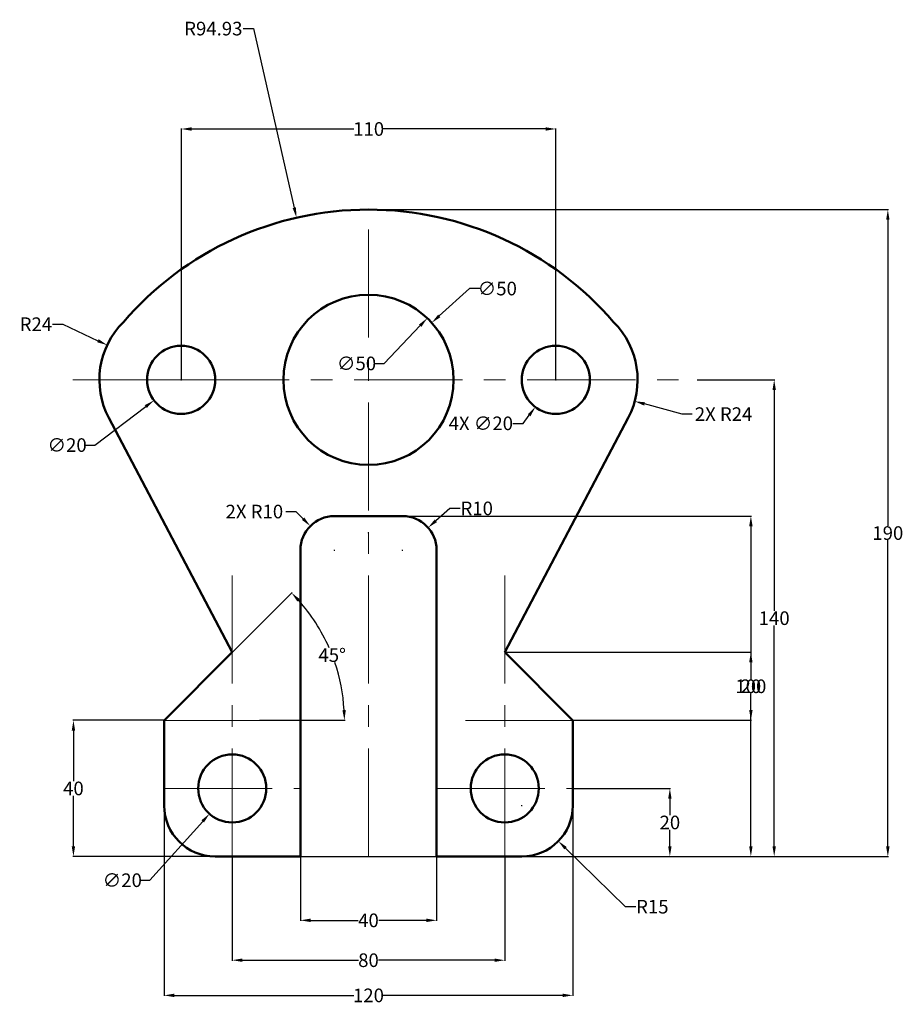
# Model space of a CAD drawing. Units: inches. Extents: x 304 to 564, y 197 to 487.
import ezdxf

# ---------------------------------------------------------------- set-up
doc = ezdxf.new("R2010")
doc.units = ezdxf.units.IN
doc.header["$MEASUREMENT"] = 0
doc.linetypes.add('CENTER', pattern=[50.8, 31.75, -6.35, 6.35, -6.35])
for name, color, linetype, lineweight in [('M-CNTR', 4, 'CENTER', 18), ('M-CONS', 8, 'Continuous', 13), ('M-DIMS', 2, 'Continuous', 25), ('M-OUTL', 7, 'Continuous', 50)]:
    doc.layers.add(name, color=color, linetype=linetype, lineweight=lineweight)
doc.styles.get("Standard").update_dxf_attribs({"font": 'arial.ttf'})
doc.dimstyles.get("Standard").update_dxf_attribs({"dimtxt": 4, "dimasz": 3, "dimexe": 0.18, "dimexo": 0.0625, "dimgap": 0.09, "dimtad": 0, "dimtih": 1, "dimtoh": 1, "dimdec": 0, "dimzin": 0, "dimdsep": 46, "dimtxsty": 'Standard', "dimcen": 0.09, "dimadec": 0, "dimazin": 0, "dimtfac": 1, "dimtdec": 0, "dimtofl": 0, "dimtmove": 0, "dimatfit": 3, "dimfxl": 1, "dimtolj": 1, "dimtzin": 0, "dimarcsym": 0})

# ---------------------------------------------------------------- blocks, each defined once
blk = doc.blocks.new('*D1')
at = {"layer": 'Defpoints', "color": 0, "transparency": 16777216}
for p in [(386.62, 240.9), (426.62, 240.9), (426.62, 222.16)]:
    blk.add_point(p, dxfattribs=at)
at = {"layer": 'M-DIMS', "color": 0, "lineweight": -2, "transparency": 16777216}
for p, q in [((386.62, 240.84), (386.62, 221.98)), ((426.62, 240.84), (426.62, 221.98)), ((389.62, 222.16), (403.6, 222.16)), ((423.62, 222.16), (409.65, 222.16))]:
    blk.add_line(p, q, dxfattribs=at)
at = {"layer": 'M-DIMS', "color": 0, "transparency": 16777216}
for points in [[(389.62, 222.66), (389.62, 221.66), (386.62, 222.16)], [(423.62, 222.66), (423.62, 221.66), (426.62, 222.16)]]:
    blk.add_solid(points, dxfattribs=at)
at = {"layer": 'M-DIMS', "color": 0, "transparency": 16777216, "insert": (406.62, 222.16), "char_height": 4, "attachment_point": 5}
blk.add_mtext('\\A1;40', dxfattribs=at)
blk = doc.blocks.new('*D2')
at = {"layer": 'Defpoints', "color": 0, "transparency": 16777216}
for p in [(392.46, 307.36), (366.62, 300.9), (346.62, 280.9), (346.62, 280.9), (374.57, 280.9)]:
    blk.add_point(p, dxfattribs=at)
at = {"layer": 'M-DIMS', "color": 0, "lineweight": -2, "transparency": 16777216}
for p, q in [((366.67, 300.94), (384.18, 318.45)), ((374.64, 280.9), (399.73, 280.9))]:
    blk.add_line(p, q, dxfattribs=at)
for start, end in [(23.6991, 41.7521), (3.2479, 18.764)]:
    blk.add_arc((346.62, 280.9), 52.93, start, end, dxfattribs=at)
at = {"layer": 'M-DIMS', "color": 0, "transparency": 16777216}
for points in [[(385.75, 315.8), (386.48, 316.49), (384.05, 318.33)], [(399.97, 283.91), (398.97, 283.88), (399.55, 280.9)]]:
    blk.add_solid(points, dxfattribs=at)
at = {"layer": 'M-DIMS', "color": 0, "transparency": 16777216, "insert": (395.97, 300.05), "char_height": 4, "attachment_point": 5}
blk.add_mtext('\\A1;45°', dxfattribs=at)
blk = doc.blocks.new('*D3')
at = {"layer": 'Defpoints', "color": 0, "transparency": 16777216}
for p in [(373.3, 268.34), (359.95, 253.45)]:
    blk.add_point(p, dxfattribs=at)
at = {"layer": 'M-DIMS', "color": 0, "lineweight": -2, "transparency": 16777216}
for p, q in [((366.53, 260.9), (366.71, 260.9)), ((366.62, 260.81), (366.62, 260.99)), ((342.47, 233.95), (357.95, 251.22)), ((339.47, 233.95), (342.47, 233.95))]:
    blk.add_line(p, q, dxfattribs=at)
at = {"layer": 'M-DIMS', "color": 0, "transparency": 16777216}
blk.add_solid([(357.57, 251.55), (358.32, 250.89), (359.95, 253.45)], dxfattribs=at)
at = {"layer": 'M-DIMS', "color": 0, "transparency": 16777216, "insert": (334.34, 233.95), "char_height": 4, "attachment_point": 5}
blk.add_mtext('\\A1;∅20', dxfattribs=at)
blk = doc.blocks.new('*D4')
at = {"layer": 'Defpoints', "color": 0, "transparency": 16777216}
for p in [(346.62, 280.9), (320, 240.9), (366.62, 240.9)]:
    blk.add_point(p, dxfattribs=at)
at = {"layer": 'M-DIMS', "color": 0, "lineweight": -2, "transparency": 16777216}
for p, q in [((346.56, 280.9), (319.82, 280.9)), ((320, 277.9), (320, 263.03)), ((320, 243.9), (320, 258.77)), ((366.56, 240.9), (319.82, 240.9))]:
    blk.add_line(p, q, dxfattribs=at)
at = {"layer": 'M-DIMS', "color": 0, "transparency": 16777216}
for points in [[(319.5, 277.9), (320.5, 277.9), (320, 280.9)], [(319.5, 243.9), (320.5, 243.9), (320, 240.9)]]:
    blk.add_solid(points, dxfattribs=at)
at = {"layer": 'M-DIMS', "color": 0, "transparency": 16777216, "insert": (320, 260.9), "char_height": 4, "attachment_point": 5}
blk.add_mtext('\\A1;40', dxfattribs=at)
blk = doc.blocks.new('*D5')
at = {"layer": 'Defpoints', "color": 0, "transparency": 16777216}
for p in [(366.62, 240.9), (446.62, 240.9), (446.62, 210.45)]:
    blk.add_point(p, dxfattribs=at)
at = {"layer": 'M-DIMS', "color": 0, "lineweight": -2, "transparency": 16777216}
for p, q in [((366.62, 240.84), (366.62, 210.27)), ((446.62, 240.84), (446.62, 210.27)), ((369.62, 210.45), (403.67, 210.45)), ((443.62, 210.45), (409.58, 210.45))]:
    blk.add_line(p, q, dxfattribs=at)
at = {"layer": 'M-DIMS', "color": 0, "transparency": 16777216}
for points in [[(369.62, 210.95), (369.62, 209.95), (366.62, 210.45)], [(443.62, 210.95), (443.62, 209.95), (446.62, 210.45)]]:
    blk.add_solid(points, dxfattribs=at)
at = {"layer": 'M-DIMS', "color": 0, "transparency": 16777216, "insert": (406.62, 210.45), "char_height": 4, "attachment_point": 5}
blk.add_mtext('\\A1;80', dxfattribs=at)
blk = doc.blocks.new('*D6')
at = {"layer": 'Defpoints', "color": 0, "transparency": 16777216}
for p in [(346.62, 255.9), (466.62, 255.9), (466.62, 200.12)]:
    blk.add_point(p, dxfattribs=at)
at = {"layer": 'M-DIMS', "color": 0, "lineweight": -2, "transparency": 16777216}
for p, q in [((346.62, 255.84), (346.62, 199.94)), ((466.62, 255.84), (466.62, 199.94)), ((349.62, 200.12), (402.31, 200.12)), ((463.62, 200.12), (410.94, 200.12))]:
    blk.add_line(p, q, dxfattribs=at)
at = {"layer": 'M-DIMS', "color": 0, "transparency": 16777216}
for points in [[(349.62, 200.62), (349.62, 199.62), (346.62, 200.12)], [(463.62, 200.62), (463.62, 199.62), (466.62, 200.12)]]:
    blk.add_solid(points, dxfattribs=at)
at = {"layer": 'M-DIMS', "color": 0, "transparency": 16777216, "insert": (406.62, 200.12), "char_height": 4, "attachment_point": 5}
blk.add_mtext('\\A1;120', dxfattribs=at)
blk = doc.blocks.new('*D7')
at = {"layer": 'Defpoints', "color": 0, "transparency": 16777216}
for p in [(423.88, 398.99), (389.37, 362.81)]:
    blk.add_point(p, dxfattribs=at)
at = {"layer": 'M-DIMS', "color": 0, "lineweight": -2, "transparency": 16777216}
for p, q in [((411.23, 385.72), (421.81, 396.82)), ((408.23, 385.72), (411.23, 385.72))]:
    blk.add_line(p, q, dxfattribs=at)
at = {"layer": 'M-DIMS', "color": 0, "transparency": 16777216}
blk.add_solid([(421.45, 397.16), (422.17, 396.47), (423.88, 398.99)], dxfattribs=at)
at = {"layer": 'M-DIMS', "color": 0, "transparency": 16777216, "insert": (403.1, 385.72), "char_height": 4, "attachment_point": 5}
blk.add_mtext('\\A1;∅50', dxfattribs=at)
blk = doc.blocks.new('*D8')
at = {"layer": 'Defpoints', "color": 0, "transparency": 16777216}
for p in [(466.62, 260.9), (451.62, 240.9), (495.1, 240.9)]:
    blk.add_point(p, dxfattribs=at)
at = {"layer": 'M-DIMS', "color": 0, "lineweight": -2, "transparency": 16777216}
for p, q in [((466.69, 260.9), (495.28, 260.9)), ((495.1, 257.9), (495.1, 253.03)), ((495.1, 243.9), (495.1, 248.77)), ((451.69, 240.9), (495.28, 240.9))]:
    blk.add_line(p, q, dxfattribs=at)
at = {"layer": 'M-DIMS', "color": 0, "transparency": 16777216}
for points in [[(494.6, 257.9), (495.6, 257.9), (495.1, 260.9)], [(494.6, 243.9), (495.6, 243.9), (495.1, 240.9)]]:
    blk.add_solid(points, dxfattribs=at)
at = {"layer": 'M-DIMS', "color": 0, "transparency": 16777216, "insert": (495.1, 250.9), "char_height": 4, "attachment_point": 5}
blk.add_mtext('\\A1;20', dxfattribs=at)
blk = doc.blocks.new('*D9')
at = {"layer": 'Defpoints', "color": 0, "transparency": 16777216}
for p in [(451.62, 255.9), (462.36, 245.42)]:
    blk.add_point(p, dxfattribs=at)
at = {"layer": 'M-DIMS', "color": 0, "lineweight": -2, "transparency": 16777216}
for p, q in [((451.53, 255.9), (451.71, 255.9)), ((451.62, 255.81), (451.62, 255.99)), ((482.07, 226.17), (464.5, 243.32)), ((485.07, 226.17), (482.07, 226.17))]:
    blk.add_line(p, q, dxfattribs=at)
at = {"layer": 'M-DIMS', "color": 0, "transparency": 16777216}
blk.add_solid([(464.85, 243.68), (464.15, 242.96), (462.36, 245.42)], dxfattribs=at)
at = {"layer": 'M-DIMS', "color": 0, "transparency": 16777216, "insert": (489.95, 226.17), "char_height": 4, "attachment_point": 5}
blk.add_mtext('\\A1;R15', dxfattribs=at)
blk = doc.blocks.new('*D10')
at = {"layer": 'Defpoints', "color": 0, "transparency": 16777216}
for p in [(406.62, 430.9), (451.62, 240.9), (559.09, 240.9)]:
    blk.add_point(p, dxfattribs=at)
at = {"layer": 'M-DIMS', "color": 0, "lineweight": -2, "transparency": 16777216}
for p, q in [((406.69, 430.9), (559.27, 430.9)), ((559.09, 427.9), (559.09, 338.03)), ((559.09, 243.9), (559.09, 333.77)), ((451.69, 240.9), (559.27, 240.9))]:
    blk.add_line(p, q, dxfattribs=at)
at = {"layer": 'M-DIMS', "color": 0, "transparency": 16777216}
for points in [[(558.59, 427.9), (559.59, 427.9), (559.09, 430.9)], [(558.59, 243.9), (559.59, 243.9), (559.09, 240.9)]]:
    blk.add_solid(points, dxfattribs=at)
at = {"layer": 'M-DIMS', "color": 0, "transparency": 16777216, "insert": (559.09, 335.9), "char_height": 4, "attachment_point": 5}
blk.add_mtext('\\A1;190', dxfattribs=at)
blk = doc.blocks.new('*D11')
at = {"layer": 'Defpoints', "color": 0, "transparency": 16777216}
for p in [(503.08, 380.9), (451.62, 240.9), (525.73, 240.9)]:
    blk.add_point(p, dxfattribs=at)
at = {"layer": 'M-DIMS', "color": 0, "lineweight": -2, "transparency": 16777216}
for p, q in [((503.14, 380.9), (525.91, 380.9)), ((525.73, 377.9), (525.73, 313.03)), ((525.73, 243.9), (525.73, 308.77)), ((451.69, 240.9), (525.91, 240.9))]:
    blk.add_line(p, q, dxfattribs=at)
at = {"layer": 'M-DIMS', "color": 0, "transparency": 16777216}
for points in [[(525.23, 377.9), (526.23, 377.9), (525.73, 380.9)], [(525.23, 243.9), (526.23, 243.9), (525.73, 240.9)]]:
    blk.add_solid(points, dxfattribs=at)
at = {"layer": 'M-DIMS', "color": 0, "transparency": 16777216, "insert": (525.73, 310.9), "char_height": 4, "attachment_point": 5}
blk.add_mtext('\\A1;140', dxfattribs=at)
blk = doc.blocks.new('*D12')
at = {"layer": 'Defpoints', "color": 0, "transparency": 16777216}
for p in [(329.9, 391.11), (351.62, 380.9)]:
    blk.add_point(p, dxfattribs=at)
at = {"layer": 'M-DIMS', "color": 0, "lineweight": -2, "transparency": 16777216}
for p, q in [((313.85, 397.24), (316.85, 397.24)), ((316.85, 397.24), (327.19, 392.38)), ((351.53, 380.9), (351.71, 380.9)), ((351.62, 380.81), (351.62, 380.99))]:
    blk.add_line(p, q, dxfattribs=at)
at = {"layer": 'M-DIMS', "color": 0, "transparency": 16777216}
blk.add_solid([(327.4, 392.84), (326.98, 391.93), (329.9, 391.11)], dxfattribs=at)
at = {"layer": 'M-DIMS', "color": 0, "transparency": 16777216, "insert": (308.99, 397.24), "char_height": 4, "attachment_point": 5}
blk.add_mtext('\\A1;R24', dxfattribs=at)
blk = doc.blocks.new('*D13')
at = {"layer": 'Defpoints', "color": 0, "transparency": 16777216}
for p in [(359.6, 386.93), (343.65, 374.87)]:
    blk.add_point(p, dxfattribs=at)
at = {"layer": 'M-DIMS', "color": 0, "lineweight": -2, "transparency": 16777216}
for p, q in [((351.53, 380.9), (351.71, 380.9)), ((351.62, 380.81), (351.62, 380.99)), ((326.27, 361.74), (341.25, 373.06)), ((323.27, 361.74), (326.27, 361.74))]:
    blk.add_line(p, q, dxfattribs=at)
at = {"layer": 'M-DIMS', "color": 0, "transparency": 16777216}
blk.add_solid([(340.95, 373.46), (341.55, 372.66), (343.65, 374.87)], dxfattribs=at)
at = {"layer": 'M-DIMS', "color": 0, "transparency": 16777216, "insert": (318.14, 361.74), "char_height": 4, "attachment_point": 5}
blk.add_mtext('\\A1;∅20', dxfattribs=at)
blk = doc.blocks.new('*D14')
at = {"layer": 'Defpoints', "color": 0, "transparency": 16777216}
for p in [(461.62, 454.57), (351.71, 380.9), (461.62, 380.9)]:
    blk.add_point(p, dxfattribs=at)
at = {"layer": 'M-DIMS', "color": 0, "lineweight": -2, "transparency": 16777216}
for p, q in [((351.71, 380.96), (351.71, 454.75)), ((354.71, 454.57), (402.36, 454.57)), ((458.62, 454.57), (410.98, 454.57)), ((461.62, 380.96), (461.62, 454.75))]:
    blk.add_line(p, q, dxfattribs=at)
at = {"layer": 'M-DIMS', "color": 0, "transparency": 16777216}
for points in [[(354.71, 455.07), (354.71, 454.07), (351.71, 454.57)], [(458.62, 455.07), (458.62, 454.07), (461.62, 454.57)]]:
    blk.add_solid(points, dxfattribs=at)
at = {"layer": 'M-DIMS', "color": 0, "transparency": 16777216, "insert": (406.67, 454.57), "char_height": 4, "attachment_point": 5}
blk.add_mtext('\\A1;110', dxfattribs=at)
blk = doc.blocks.new('*D15')
at = {"layer": 'Defpoints', "color": 0, "transparency": 16777216}
for p in [(424.13, 337.5), (416.62, 330.9)]:
    blk.add_point(p, dxfattribs=at)
at = {"layer": 'M-DIMS', "color": 0, "lineweight": -2, "transparency": 16777216}
for p, q in [((430.54, 343.14), (426.38, 339.49)), ((433.54, 343.14), (430.54, 343.14)), ((416.53, 330.9), (416.71, 330.9)), ((416.62, 330.81), (416.62, 330.99))]:
    blk.add_line(p, q, dxfattribs=at)
at = {"layer": 'M-DIMS', "color": 0, "transparency": 16777216}
blk.add_solid([(426.05, 339.86), (426.71, 339.11), (424.13, 337.5)], dxfattribs=at)
at = {"layer": 'M-DIMS', "color": 0, "transparency": 16777216, "insert": (438.4, 343.14), "char_height": 4, "attachment_point": 5}
blk.add_mtext('\\A1;R10', dxfattribs=at)
blk = doc.blocks.new('MOUNT-HOLE-D20')
blk.add_circle((10, 10), 10)
blk = doc.blocks.new('*D17')
at = {"layer": 'Defpoints', "color": 0, "transparency": 16777216}
for p in [(446.62, 300.9), (518.88, 300.9), (466.62, 280.9)]:
    blk.add_point(p, dxfattribs=at)
at = {"layer": 'M-DIMS', "color": 0, "lineweight": -2, "transparency": 16777216}
for p, q in [((446.69, 300.9), (519.06, 300.9)), ((518.88, 297.9), (518.88, 293.03)), ((518.88, 283.9), (518.88, 288.77)), ((466.69, 280.9), (519.06, 280.9))]:
    blk.add_line(p, q, dxfattribs=at)
at = {"layer": 'M-DIMS', "color": 0, "transparency": 16777216}
for points in [[(518.38, 297.9), (519.38, 297.9), (518.88, 300.9)], [(518.38, 283.9), (519.38, 283.9), (518.88, 280.9)]]:
    blk.add_solid(points, dxfattribs=at)
at = {"layer": 'M-DIMS', "color": 0, "transparency": 16777216, "insert": (518.88, 290.9), "char_height": 4, "attachment_point": 5}
blk.add_mtext('\\A1;20', dxfattribs=at)
blk = doc.blocks.new('*D18')
at = {"layer": 'Defpoints', "color": 0, "transparency": 16777216}
for p in [(396.62, 340.9), (518.88, 340.9), (386.62, 240.9)]:
    blk.add_point(p, dxfattribs=at)
at = {"layer": 'M-DIMS', "color": 0, "lineweight": -2, "transparency": 16777216}
for p, q in [((396.69, 340.9), (519.06, 340.9)), ((518.88, 337.9), (518.88, 293.03)), ((518.88, 243.9), (518.88, 288.77)), ((386.69, 240.9), (519.06, 240.9))]:
    blk.add_line(p, q, dxfattribs=at)
at = {"layer": 'M-DIMS', "color": 0, "transparency": 16777216}
for points in [[(518.38, 337.9), (519.38, 337.9), (518.88, 340.9)], [(518.38, 243.9), (519.38, 243.9), (518.88, 240.9)]]:
    blk.add_solid(points, dxfattribs=at)
at = {"layer": 'M-DIMS', "color": 0, "transparency": 16777216, "insert": (518.88, 290.9), "char_height": 4, "attachment_point": 5}
blk.add_mtext('\\A1;100', dxfattribs=at)
blk = doc.blocks.new('*D19')
at = {"layer": 'Defpoints', "color": 0, "transparency": 16777216}
for p in [(385.5, 428.52), (406.62, 335.97)]:
    blk.add_point(p, dxfattribs=at)
at = {"layer": 'M-DIMS', "color": 0, "lineweight": -2, "transparency": 16777216}
for p, q in [((369.83, 484.05), (372.83, 484.05)), ((372.83, 484.05), (384.83, 431.44)), ((406.53, 335.97), (406.71, 335.97)), ((406.62, 335.88), (406.62, 336.06))]:
    blk.add_line(p, q, dxfattribs=at)
at = {"layer": 'M-DIMS', "color": 0, "transparency": 16777216}
blk.add_solid([(385.32, 431.55), (384.35, 431.33), (385.5, 428.52)], dxfattribs=at)
at = {"layer": 'M-DIMS', "color": 0, "transparency": 16777216, "insert": (361.07, 484.05), "char_height": 4, "attachment_point": 5}
blk.add_mtext('\\A1;R94.93', dxfattribs=at)
blk = doc.blocks.new('*D20')
at = {"layer": 'Defpoints', "color": 0, "transparency": 16777216}
for p in [(461.62, 380.9), (484.78, 374.6)]:
    blk.add_point(p, dxfattribs=at)
at = {"layer": 'M-DIMS', "color": 0, "lineweight": -2, "transparency": 16777216}
for p, q in [((461.53, 380.9), (461.71, 380.9)), ((461.62, 380.81), (461.62, 380.99)), ((498.68, 370.83), (487.68, 373.82)), ((501.68, 370.83), (498.68, 370.83))]:
    blk.add_line(p, q, dxfattribs=at)
at = {"layer": 'M-DIMS', "color": 0, "transparency": 16777216}
blk.add_solid([(487.81, 374.3), (487.55, 373.33), (484.78, 374.6)], dxfattribs=at)
at = {"layer": 'M-DIMS', "color": 0, "transparency": 16777216, "insert": (510.87, 370.83), "char_height": 4, "attachment_point": 5}
blk.add_mtext('\\A1;2X R24', dxfattribs=at)
blk = doc.blocks.new('*D21')
at = {"layer": 'Defpoints', "color": 0, "transparency": 16777216}
for p in [(389.55, 337.97), (396.62, 330.9)]:
    blk.add_point(p, dxfattribs=at)
at = {"layer": 'M-DIMS', "color": 0, "lineweight": -2, "transparency": 16777216}
for p, q in [((382.31, 342.21), (385.31, 342.21)), ((385.31, 342.21), (387.43, 340.09)), ((396.53, 330.9), (396.71, 330.9)), ((396.62, 330.81), (396.62, 330.99))]:
    blk.add_line(p, q, dxfattribs=at)
at = {"layer": 'M-DIMS', "color": 0, "transparency": 16777216}
blk.add_solid([(387.79, 340.44), (387.08, 339.74), (389.55, 337.97)], dxfattribs=at)
at = {"layer": 'M-DIMS', "color": 0, "transparency": 16777216, "insert": (373.12, 342.21), "char_height": 4, "attachment_point": 5}
blk.add_mtext('\\A1;2X R10', dxfattribs=at)
blk = doc.blocks.new('*D22')
at = {"layer": 'Defpoints', "color": 0, "transparency": 16777216}
for p in [(467.64, 388.89), (455.61, 372.91)]:
    blk.add_point(p, dxfattribs=at)
at = {"layer": 'M-DIMS', "color": 0, "lineweight": -2, "transparency": 16777216}
for p, q in [((461.53, 380.9), (461.71, 380.9)), ((461.62, 380.81), (461.62, 380.99)), ((452, 368.12), (453.8, 370.51)), ((449, 368.12), (452, 368.12))]:
    blk.add_line(p, q, dxfattribs=at)
at = {"layer": 'M-DIMS', "color": 0, "transparency": 16777216}
blk.add_solid([(453.4, 370.82), (454.2, 370.21), (455.61, 372.91)], dxfattribs=at)
at = {"layer": 'M-DIMS', "color": 0, "transparency": 16777216, "insert": (439.6, 368.12), "char_height": 4, "attachment_point": 5}
blk.add_mtext('\\A1;4X ∅20', dxfattribs=at)
blk = doc.blocks.new('*D23')
at = {"layer": 'Defpoints', "color": 0, "transparency": 16777216}
for p in [(425.18, 397.66), (388.07, 364.14)]:
    blk.add_point(p, dxfattribs=at)
at = {"layer": 'M-DIMS', "color": 0, "lineweight": -2, "transparency": 16777216}
for p, q in [((436.31, 407.71), (427.4, 399.67)), ((439.31, 407.71), (436.31, 407.71)), ((406.53, 380.9), (406.71, 380.9)), ((406.62, 380.81), (406.62, 380.99))]:
    blk.add_line(p, q, dxfattribs=at)
at = {"layer": 'M-DIMS', "color": 0, "transparency": 16777216}
blk.add_solid([(427.07, 400.04), (427.74, 399.3), (425.18, 397.66)], dxfattribs=at)
at = {"layer": 'M-DIMS', "color": 0, "transparency": 16777216, "insert": (444.43, 407.71), "char_height": 4, "attachment_point": 5}
blk.add_mtext('\\A1;∅50', dxfattribs=at)

msp = doc.modelspace()

# ---------------------------------------------------------------- linework, layer by layer
at = {"layer": 'M-CNTR'}
for p, q in [((406.624, 240.899), (406.624, 430.899)), ((351.624, 380.899), (315.879, 380.899)), ((351.624, 380.899), (503.082, 380.899)), ((446.624, 240.899), (446.624, 327.03)), ((366.624, 240.899), (366.624, 326.046)), ((346.624, 260.899), (386.624, 260.899)), ((426.624, 260.899), (466.624, 260.899))]:
    msp.add_line(p, q, dxfattribs=at)
at = {"layer": 'M-CONS'}
for p, q in [((346.624, 280.899), (374.573, 280.899)), ((466.624, 280.899), (435.11, 280.899)), ((426.624, 240.899), (406.624, 240.899))]:
    msp.add_line(p, q, dxfattribs=at)
at = {"layer": 'M-OUTL'}
for p, q in [((366.624, 300.899), (330.388, 369.717)), ((446.624, 300.899), (482.861, 369.717)), ((396.624, 340.899), (416.624, 340.899)), ((386.624, 240.899), (386.624, 330.899)), ((426.624, 330.899), (426.624, 240.899)), ((346.624, 280.899), (366.624, 300.899)), ((466.624, 280.899), (446.624, 300.899)), ((346.624, 255.899), (346.624, 280.899)), ((466.624, 255.899), (466.624, 280.899)), ((386.624, 240.899), (361.624, 240.899)), ((426.624, 240.899), (451.624, 240.899))]:
    msp.add_line(p, q, dxfattribs=at)
msp.add_circle((406.624, 380.899), 25, dxfattribs=at)
for centre, radius, start, end in [((406.624, 335.973), 94.926, 40.6964, 139.3036), ((351.624, 380.899), 24, 135, 207.7689), ((461.624, 380.899), 24, 332.2311, 45), ((396.624, 330.899), 10, 90, 180), ((416.624, 330.899), 10, 0, 90), ((361.624, 255.899), 15, 180, 270), ((451.624, 255.899), 15, 270, 0)]:
    msp.add_arc(centre, radius, start, end, dxfattribs=at)

# ---------------------------------------------------------------- block references
for p in [(341.624, 370.899), (451.624, 370.899), (356.624, 250.899), (436.624, 250.899)]:
    msp.add_blockref('MOUNT-HOLE-D20', p, dxfattribs=at)

# ---------------------------------------------------------------- dimensions: what is measured, and where the dimension line sits
at = {"layer": 'M-DIMS'}
for center, mpoint, override, picture, middle in [((406.624, 335.973), (385.5, 428.519), {"dimdec": 2, "dimlfac": 1, "dimrnd": 0, "dimzin": 0, "dimdsep": 46, "dimlunit": 2}, '*D19', (361.073, 484.046)), ((351.624, 380.899), (329.904, 391.107), {"dimclrd": 0, "dimclre": 0, "dimclrt": 0}, '*D12', (308.989, 397.243)), ((416.624, 330.899), (424.132, 337.505), {"dimclrd": 0, "dimclre": 0, "dimclrt": 0}, '*D15', (438.403, 343.144)), ((451.624, 255.899), (462.356, 245.419), {"dimclrd": 0, "dimclre": 0, "dimclrt": 0}, '*D9', (489.952, 226.167))]:
    dim = msp.add_radius_dim(center=center, mpoint=mpoint, dimstyle='Standard', override=override, dxfattribs=at)
    dim.commit()
    dim.dimension.update_dxf_attribs({"geometry": picture, "text_midpoint": middle, "dimtype": 164})
dim = msp.add_linear_dim(base=(461.624, 454.566), p1=(351.714, 380.899), p2=(461.624, 380.899), dimstyle='Standard', override={"dimclrd": 0, "dimclre": 0, "dimclrt": 0}, dxfattribs=at)
dim.commit()
dim.dimension.update_dxf_attribs({"geometry": '*D14', "text_midpoint": (406.669, 454.566)})
for base, p1, p2, override, picture, middle in [((559.088, 240.899), (406.624, 430.899), (451.624, 240.899), {"dimclrd": 0, "dimclre": 0, "dimclrt": 0}, '*D10', (559.088, 335.899)), ((525.728, 240.899), (503.082, 380.899), (451.624, 240.899), {"dimclrd": 0, "dimclre": 0, "dimclrt": 0}, '*D11', (525.728, 310.899)), ((518.882, 340.899), (386.624, 240.899), (396.624, 340.899), {"dimdec": 0, "dimlfac": 1, "dimrnd": 0, "dimzin": 0, "dimdsep": 46, "dimlunit": 2}, '*D18', (518.882, 290.899)), ((518.882, 300.899), (466.624, 280.899), (446.624, 300.899), {"dimdec": 0, "dimlfac": 1, "dimrnd": 0, "dimzin": 0, "dimdsep": 46, "dimlunit": 2}, '*D17', (518.882, 290.899)), ((320.002, 240.899), (346.624, 280.899), (366.624, 240.899), {"dimclrd": 0, "dimclre": 0, "dimclrt": 0}, '*D4', (320.002, 260.899)), ((495.102, 240.899), (466.624, 260.899), (451.624, 240.899), {"dimclrd": 0, "dimclre": 0, "dimclrt": 0}, '*D8', (495.102, 250.899))]:
    dim = msp.add_linear_dim(base=base, p1=p1, p2=p2, angle=90, dimstyle='Standard', override=override, dxfattribs=at)
    dim.commit()
    dim.dimension.update_dxf_attribs({"geometry": picture, "text_midpoint": middle})
for p1, p2, override, picture, middle in [((388.074, 364.14), (425.175, 397.658), {"dimdec": 0, "dimlfac": 1, "dimrnd": 0, "dimzin": 0, "dimdsep": 46, "dimlunit": 2}, '*D23', (444.43, 407.714)), ((389.368, 362.81), (423.881, 398.988), {"dimclrd": 0, "dimclre": 0, "dimclrt": 0}, '*D7', (403.102, 385.722)), ((359.604, 386.926), (343.645, 374.871), {"dimclrd": 0, "dimclre": 0, "dimclrt": 0}, '*D13', (318.144, 361.745)), ((373.3, 268.345), (359.949, 253.453), {"dimclrd": 0, "dimclre": 0, "dimclrt": 0}, '*D3', (334.342, 233.95))]:
    dim = msp.add_diameter_dim_2p(p1=p1, p2=p2, dimstyle='Standard', override=override, dxfattribs=at)
    dim.commit()
    dim.dimension.update_dxf_attribs({"geometry": picture, "text_midpoint": middle, "dimtype": 163})
dim = msp.add_diameter_dim_2p(p1=(467.641, 388.887), p2=(455.608, 372.911), text='4X <>', dimstyle='Standard', override={"dimdec": 0, "dimlfac": 1, "dimrnd": 0, "dimzin": 0, "dimdsep": 46, "dimlunit": 2}, dxfattribs=at)
dim.commit()
dim.dimension.update_dxf_attribs({"geometry": '*D22', "text_midpoint": (439.603, 368.118), "dimtype": 163})
for center, mpoint, picture, middle in [((461.624, 380.899), (484.784, 374.604), '*D20', (510.873, 370.827)), ((396.624, 330.899), (389.553, 337.97), '*D21', (373.117, 342.212))]:
    dim = msp.add_radius_dim(center=center, mpoint=mpoint, text='2X <>', dimstyle='Standard', override={"dimdec": 0, "dimlfac": 1, "dimrnd": 0, "dimzin": 0, "dimdsep": 46, "dimlunit": 2}, dxfattribs=at)
    dim.commit()
    dim.dimension.update_dxf_attribs({"geometry": picture, "text_midpoint": middle, "dimtype": 164})
dim = msp.add_angular_dim_2l(base=(392.463, 307.364), line1=((346.624, 280.899), (374.573, 280.899)), line2=((346.624, 280.899), (366.624, 300.899)), dimstyle='Standard', override={"dimclrd": 0, "dimclre": 0, "dimclrt": 0}, dxfattribs=at)
dim.commit()
dim.dimension.update_dxf_attribs({"geometry": '*D2', "text_midpoint": (395.968, 300.049), "dimtype": 162})
for base, p1, p2, picture, middle in [((466.624, 200.123), (346.624, 255.899), (466.624, 255.899), '*D6', (406.624, 200.123)), ((446.624, 210.454), (366.624, 240.899), (446.624, 240.899), '*D5', (406.624, 210.454))]:
    dim = msp.add_linear_dim(base=base, p1=p1, p2=p2, dimstyle='Standard', override={"dimclrd": 0, "dimclre": 0, "dimclrt": 0}, dxfattribs=at)
    dim.commit()
    dim.dimension.update_dxf_attribs({"geometry": picture, "text_midpoint": middle, "dimtype": 160})
dim = msp.add_linear_dim(base=(426.624, 222.162), p1=(386.624, 240.899), p2=(426.624, 240.899), angle=180, dimstyle='Standard', override={"dimclrd": 0, "dimclre": 0, "dimclrt": 0}, dxfattribs=at)
dim.commit()
dim.dimension.update_dxf_attribs({"geometry": '*D1', "text_midpoint": (406.624, 222.162), "dimtype": 160})

doc.saveas('drawing.dxf')
